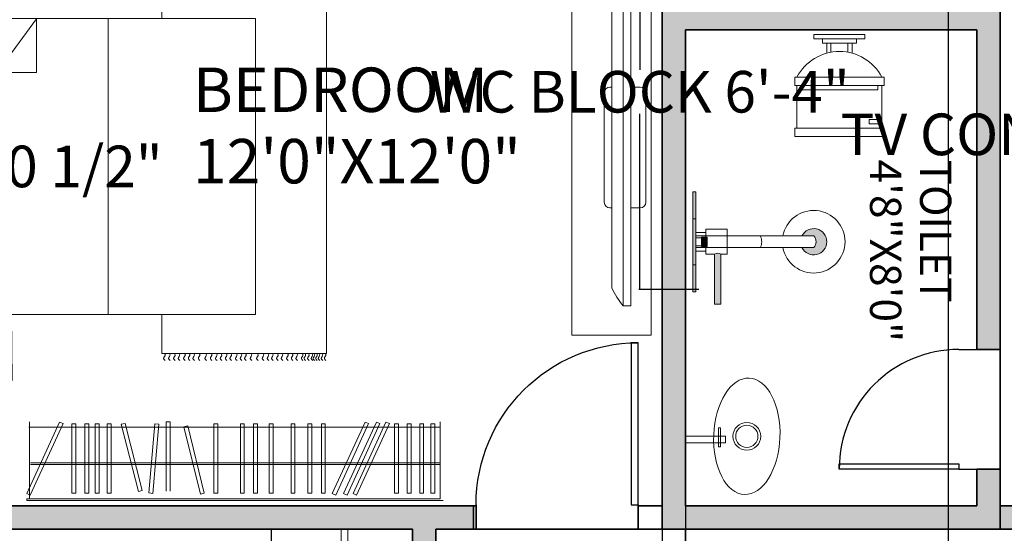
# Model space of a CAD drawing. Units: inches. Extents: x -4737294 to -4736756, y 1716389 to 1717040.
# Tile 20 of 25: x -4737186 to -4736996, y 1716844 to 1716943. Entities that reach past the tile are written whole.
import ezdxf

# ---------------------------------------------------------------- set-up
doc = ezdxf.new("R2010")
doc.units = ezdxf.units.IN
doc.header["$MEASUREMENT"] = 0
for name, color, linetype, lineweight in [('A-ANNO-DIMS', 2, 'Continuous', 18), ('A-AREA-IDEN', 250, 'Continuous', 18), ('A-WALL-PATT', 244, 'Continuous', 13), ('closet', 252, 'Continuous', 18), ('doors', 252, 'Continuous', 25), ('furniture', 250, 'Continuous', 18), ('PLUMBING FIXTURES', 252, 'Continuous', 18), ('walls', 252, 'Continuous', 35)]:
    doc.layers.add(name, color=color, linetype=linetype, lineweight=lineweight)
doc.styles.get("Standard").update_dxf_attribs({"font": 'arial.ttf'})
doc.dimstyles.get("Standard").update_dxf_attribs({"dimtxt": 8, "dimasz": 0.18, "dimexe": 0.18, "dimexo": 0.0625, "dimgap": 0.09, "dimtad": 0, "dimtih": 1, "dimtoh": 1, "dimzin": 0, "dimdsep": 46, "dimlunit": 3, "dimtxsty": 'Standard', "dimcen": 0.09, "dimadec": 0, "dimazin": 0, "dimtfac": 1, "dimtofl": 0, "dimtmove": 0, "dimatfit": 3, "dimfxl": 1, "dimtolj": 1, "dimtzin": 0, "dimarcsym": 0})

# ---------------------------------------------------------------- blocks, each defined once
blk = doc.blocks.new('CARPET')
at = {"layer": 'furniture'}
for p, q in [((-51.53, -98.11), (-51.53, -55.12)), ((-51.53, -55.12), (-41.27, -55.12)), ((36, -55.12), (51.55, -55.12)), ((51.55, -55.12), (51.55, -98.11)), ((51.55, -98.11), (-51.53, -98.11))]:
    blk.add_line(p, q, dxfattribs=at)
for points, knots in [([(-53.37, -55.99), (-53.22, -55.8), (-52.9, -55.41), (-52.34, -55.8), (-51.89, -56.08), (-51.65, -55.91), (-51.53, -55.83)], [0, 0, 0, 0, 0.653278, 1.290138, 1.740457, 2.114451, 2.114451, 2.114451, 2.114451]), ([(53.37, -55.99), (53.22, -55.8), (52.9, -55.41), (52.34, -55.8), (51.89, -56.08), (51.65, -55.91), (51.53, -55.83)], [0, 0, 0, 0, 0.653278, 1.290138, 1.740457, 2.114451, 2.114451, 2.114451, 2.114451]), ([(-53.37, -57.26), (-53.22, -57.07), (-52.9, -56.67), (-52.34, -57.07), (-51.89, -57.35), (-51.65, -57.17), (-51.53, -57.1)], [0, 0, 0, 0, 0.653278, 1.290138, 1.740457, 2.114451, 2.114451, 2.114451, 2.114451]), ([(-53.37, -58.59), (-53.22, -58.4), (-52.9, -58.01), (-52.34, -58.4), (-51.89, -58.68), (-51.65, -58.5), (-51.53, -58.43)], [0, 0, 0, 0, 0.653278, 1.290138, 1.740457, 2.114451, 2.114451, 2.114451, 2.114451]), ([(53.37, -57.26), (53.22, -57.07), (52.9, -56.67), (52.34, -57.07), (51.89, -57.35), (51.65, -57.17), (51.53, -57.1)], [0, 0, 0, 0, 0.653278, 1.290138, 1.740457, 2.114451, 2.114451, 2.114451, 2.114451]), ([(53.37, -58.59), (53.22, -58.4), (52.9, -58.01), (52.34, -58.4), (51.89, -58.68), (51.65, -58.5), (51.53, -58.43)], [0, 0, 0, 0, 0.653278, 1.290138, 1.740457, 2.114451, 2.114451, 2.114451, 2.114451]), ([(-53.37, -59.78), (-53.22, -59.58), (-52.9, -59.19), (-52.34, -59.58), (-51.89, -59.86), (-51.65, -59.69), (-51.53, -59.61)], [0, 0, 0, 0, 0.653278, 1.290138, 1.740457, 2.114451, 2.114451, 2.114451, 2.114451]), ([(-53.37, -61.22), (-53.22, -61.02), (-52.9, -60.63), (-52.34, -61.02), (-51.89, -61.3), (-51.65, -61.13), (-51.53, -61.05)], [0, 0, 0, 0, 0.653278, 1.290138, 1.740457, 2.114451, 2.114451, 2.114451, 2.114451]), ([(53.37, -59.78), (53.22, -59.58), (52.9, -59.19), (52.34, -59.58), (51.89, -59.86), (51.65, -59.69), (51.53, -59.61)], [0, 0, 0, 0, 0.653278, 1.290138, 1.740457, 2.114451, 2.114451, 2.114451, 2.114451]), ([(53.37, -61.22), (53.22, -61.02), (52.9, -60.63), (52.34, -61.02), (51.89, -61.3), (51.65, -61.13), (51.53, -61.05)], [0, 0, 0, 0, 0.653278, 1.290138, 1.740457, 2.114451, 2.114451, 2.114451, 2.114451]), ([(-53.37, -62.44), (-53.22, -62.25), (-52.9, -61.86), (-52.34, -62.25), (-51.89, -62.53), (-51.65, -62.36), (-51.53, -62.28)], [0, 0, 0, 0, 0.653278, 1.290138, 1.740457, 2.114451, 2.114451, 2.114451, 2.114451]), ([(-53.37, -63.63), (-53.22, -63.43), (-52.9, -63.04), (-52.34, -63.43), (-51.89, -63.72), (-51.65, -63.54), (-51.53, -63.46)], [0, 0, 0, 0, 0.653278, 1.290138, 1.740457, 2.114451, 2.114451, 2.114451, 2.114451]), ([(53.37, -62.44), (53.22, -62.25), (52.9, -61.86), (52.34, -62.25), (51.89, -62.53), (51.65, -62.36), (51.53, -62.28)], [0, 0, 0, 0, 0.653278, 1.290138, 1.740457, 2.114451, 2.114451, 2.114451, 2.114451]), ([(53.37, -63.63), (53.22, -63.43), (52.9, -63.04), (52.34, -63.43), (51.89, -63.72), (51.65, -63.54), (51.53, -63.46)], [0, 0, 0, 0, 0.653278, 1.290138, 1.740457, 2.114451, 2.114451, 2.114451, 2.114451]), ([(-53.37, -65.07), (-53.22, -64.87), (-52.9, -64.48), (-52.34, -64.87), (-51.89, -65.15), (-51.65, -64.98), (-51.53, -64.9)], [0, 0, 0, 0, 0.653278, 1.290138, 1.740457, 2.114451, 2.114451, 2.114451, 2.114451]), ([(-53.37, -66.76), (-53.22, -66.56), (-52.9, -66.17), (-52.34, -66.56), (-51.89, -66.84), (-51.65, -66.67), (-51.53, -66.59)], [0, 0, 0, 0, 0.653278, 1.290138, 1.740457, 2.114451, 2.114451, 2.114451, 2.114451]), ([(53.37, -65.07), (53.22, -64.87), (52.9, -64.48), (52.34, -64.87), (51.89, -65.15), (51.65, -64.98), (51.53, -64.9)], [0, 0, 0, 0, 0.653278, 1.290138, 1.740457, 2.114451, 2.114451, 2.114451, 2.114451]), ([(53.37, -66.76), (53.22, -66.56), (52.9, -66.17), (52.34, -66.56), (51.89, -66.84), (51.65, -66.67), (51.53, -66.59)], [0, 0, 0, 0, 0.653278, 1.290138, 1.740457, 2.114451, 2.114451, 2.114451, 2.114451]), ([(-53.37, -68.2), (-53.22, -68), (-52.9, -67.61), (-52.34, -68), (-51.89, -68.28), (-51.65, -68.11), (-51.53, -68.03)], [0, 0, 0, 0, 0.653278, 1.290138, 1.740457, 2.114451, 2.114451, 2.114451, 2.114451]), ([(-53.37, -69.53), (-53.22, -69.33), (-52.9, -68.94), (-52.34, -69.33), (-51.89, -69.61), (-51.65, -69.44), (-51.53, -69.36)], [0, 0, 0, 0, 0.653278, 1.290138, 1.740457, 2.114451, 2.114451, 2.114451, 2.114451]), ([(53.37, -68.2), (53.22, -68), (52.9, -67.61), (52.34, -68), (51.89, -68.28), (51.65, -68.11), (51.53, -68.03)], [0, 0, 0, 0, 0.653278, 1.290138, 1.740457, 2.114451, 2.114451, 2.114451, 2.114451]), ([(53.37, -69.53), (53.22, -69.33), (52.9, -68.94), (52.34, -69.33), (51.89, -69.61), (51.65, -69.44), (51.53, -69.36)], [0, 0, 0, 0, 0.653278, 1.290138, 1.740457, 2.114451, 2.114451, 2.114451, 2.114451]), ([(-53.37, -70.79), (-53.22, -70.6), (-52.9, -70.21), (-52.34, -70.6), (-51.89, -70.88), (-51.65, -70.7), (-51.53, -70.63)], [0, 0, 0, 0, 0.653278, 1.290138, 1.740457, 2.114451, 2.114451, 2.114451, 2.114451]), ([(-53.37, -72.12), (-53.22, -71.93), (-52.9, -71.54), (-52.34, -71.93), (-51.89, -72.21), (-51.65, -72.04), (-51.53, -71.96)], [0, 0, 0, 0, 0.653278, 1.290138, 1.740457, 2.114451, 2.114451, 2.114451, 2.114451]), ([(53.37, -70.79), (53.22, -70.6), (52.9, -70.21), (52.34, -70.6), (51.89, -70.88), (51.65, -70.7), (51.53, -70.63)], [0, 0, 0, 0, 0.653278, 1.290138, 1.740457, 2.114451, 2.114451, 2.114451, 2.114451]), ([(53.37, -72.12), (53.22, -71.93), (52.9, -71.54), (52.34, -71.93), (51.89, -72.21), (51.65, -72.04), (51.53, -71.96)], [0, 0, 0, 0, 0.653278, 1.290138, 1.740457, 2.114451, 2.114451, 2.114451, 2.114451]), ([(-53.37, -73.31), (-53.22, -73.11), (-52.9, -72.72), (-52.34, -73.11), (-51.89, -73.4), (-51.65, -73.22), (-51.53, -73.14)], [0, 0, 0, 0, 0.653278, 1.290138, 1.740457, 2.114451, 2.114451, 2.114451, 2.114451]), ([(-53.37, -74.75), (-53.22, -74.55), (-52.9, -74.16), (-52.34, -74.55), (-51.89, -74.83), (-51.65, -74.66), (-51.53, -74.58)], [0, 0, 0, 0, 0.653278, 1.290138, 1.740457, 2.114451, 2.114451, 2.114451, 2.114451]), ([(53.37, -73.31), (53.22, -73.11), (52.9, -72.72), (52.34, -73.11), (51.89, -73.4), (51.65, -73.22), (51.53, -73.14)], [0, 0, 0, 0, 0.653278, 1.290138, 1.740457, 2.114451, 2.114451, 2.114451, 2.114451]), ([(53.37, -74.75), (53.22, -74.55), (52.9, -74.16), (52.34, -74.55), (51.89, -74.83), (51.65, -74.66), (51.53, -74.58)], [0, 0, 0, 0, 0.653278, 1.290138, 1.740457, 2.114451, 2.114451, 2.114451, 2.114451]), ([(-53.37, -75.98), (-53.22, -75.78), (-52.9, -75.39), (-52.34, -75.78), (-51.89, -76.06), (-51.65, -75.89), (-51.53, -75.81)], [0, 0, 0, 0, 0.653278, 1.290138, 1.740457, 2.114451, 2.114451, 2.114451, 2.114451]), ([(-53.37, -77.16), (-53.22, -76.96), (-52.9, -76.57), (-52.34, -76.96), (-51.89, -77.25), (-51.65, -77.07), (-51.53, -76.99)], [0, 0, 0, 0, 0.653278, 1.290138, 1.740457, 2.114451, 2.114451, 2.114451, 2.114451]), ([(53.37, -75.98), (53.22, -75.78), (52.9, -75.39), (52.34, -75.78), (51.89, -76.06), (51.65, -75.89), (51.53, -75.81)], [0, 0, 0, 0, 0.653278, 1.290138, 1.740457, 2.114451, 2.114451, 2.114451, 2.114451]), ([(53.37, -77.16), (53.22, -76.96), (52.9, -76.57), (52.34, -76.96), (51.89, -77.25), (51.65, -77.07), (51.53, -76.99)], [0, 0, 0, 0, 0.653278, 1.290138, 1.740457, 2.114451, 2.114451, 2.114451, 2.114451]), ([(-53.37, -78.6), (-53.22, -78.4), (-52.9, -78.01), (-52.34, -78.4), (-51.89, -78.68), (-51.65, -78.51), (-51.53, -78.43)], [0, 0, 0, 0, 0.653278, 1.290138, 1.740457, 2.114451, 2.114451, 2.114451, 2.114451]), ([(53.37, -78.6), (53.22, -78.4), (52.9, -78.01), (52.34, -78.4), (51.89, -78.68), (51.65, -78.51), (51.53, -78.43)], [0, 0, 0, 0, 0.653278, 1.290138, 1.740457, 2.114451, 2.114451, 2.114451, 2.114451]), ([(-53.37, -80.29), (-53.22, -80.09), (-52.9, -79.7), (-52.34, -80.09), (-51.89, -80.37), (-51.65, -80.2), (-51.53, -80.12)], [0, 0, 0, 0, 0.653278, 1.290138, 1.740457, 2.114451, 2.114451, 2.114451, 2.114451]), ([(-53.37, -81.73), (-53.22, -81.53), (-52.9, -81.14), (-52.34, -81.53), (-51.89, -81.81), (-51.65, -81.64), (-51.53, -81.56)], [0, 0, 0, 0, 0.653278, 1.290138, 1.740457, 2.114451, 2.114451, 2.114451, 2.114451]), ([(53.37, -80.29), (53.22, -80.09), (52.9, -79.7), (52.34, -80.09), (51.89, -80.37), (51.65, -80.2), (51.53, -80.12)], [0, 0, 0, 0, 0.653278, 1.290138, 1.740457, 2.114451, 2.114451, 2.114451, 2.114451]), ([(53.37, -81.73), (53.22, -81.53), (52.9, -81.14), (52.34, -81.53), (51.89, -81.81), (51.65, -81.64), (51.53, -81.56)], [0, 0, 0, 0, 0.653278, 1.290138, 1.740457, 2.114451, 2.114451, 2.114451, 2.114451]), ([(-53.37, -83.06), (-53.22, -82.86), (-52.9, -82.47), (-52.34, -82.86), (-51.89, -83.14), (-51.65, -82.97), (-51.53, -82.89)], [0, 0, 0, 0, 0.653278, 1.290138, 1.740457, 2.114451, 2.114451, 2.114451, 2.114451]), ([(-53.37, -84.18), (-53.22, -83.99), (-52.9, -83.6), (-52.34, -83.99), (-51.89, -84.27), (-51.65, -84.09), (-51.53, -84.02)], [0, 0, 0, 0, 0.653278, 1.290138, 1.740457, 2.114451, 2.114451, 2.114451, 2.114451]), ([(53.37, -83.06), (53.22, -82.86), (52.9, -82.47), (52.34, -82.86), (51.89, -83.14), (51.65, -82.97), (51.53, -82.89)], [0, 0, 0, 0, 0.653278, 1.290138, 1.740457, 2.114451, 2.114451, 2.114451, 2.114451]), ([(53.37, -84.18), (53.22, -83.99), (52.9, -83.6), (52.34, -83.99), (51.89, -84.27), (51.65, -84.09), (51.53, -84.02)], [0, 0, 0, 0, 0.653278, 1.290138, 1.740457, 2.114451, 2.114451, 2.114451, 2.114451]), ([(-53.37, -85.51), (-53.22, -85.32), (-52.9, -84.93), (-52.34, -85.32), (-51.89, -85.6), (-51.65, -85.42), (-51.53, -85.35)], [0, 0, 0, 0, 0.653278, 1.290138, 1.740457, 2.114451, 2.114451, 2.114451, 2.114451]), ([(-53.37, -86.7), (-53.22, -86.5), (-52.9, -86.11), (-52.34, -86.5), (-51.89, -86.78), (-51.65, -86.61), (-51.53, -86.53)], [0, 0, 0, 0, 0.653278, 1.290138, 1.740457, 2.114451, 2.114451, 2.114451, 2.114451]), ([(53.37, -85.51), (53.22, -85.32), (52.9, -84.93), (52.34, -85.32), (51.89, -85.6), (51.65, -85.42), (51.53, -85.35)], [0, 0, 0, 0, 0.653278, 1.290138, 1.740457, 2.114451, 2.114451, 2.114451, 2.114451]), ([(53.37, -86.7), (53.22, -86.5), (52.9, -86.11), (52.34, -86.5), (51.89, -86.78), (51.65, -86.61), (51.53, -86.53)], [0, 0, 0, 0, 0.653278, 1.290138, 1.740457, 2.114451, 2.114451, 2.114451, 2.114451]), ([(-53.37, -88.14), (-53.22, -87.94), (-52.9, -87.55), (-52.34, -87.94), (-51.89, -88.22), (-51.65, -88.05), (-51.53, -87.97)], [0, 0, 0, 0, 0.653278, 1.290138, 1.740457, 2.114451, 2.114451, 2.114451, 2.114451]), ([(-53.37, -89.36), (-53.22, -89.17), (-52.9, -88.78), (-52.34, -89.17), (-51.89, -89.45), (-51.65, -89.28), (-51.53, -89.2)], [0, 0, 0, 0, 0.653278, 1.290138, 1.740457, 2.114451, 2.114451, 2.114451, 2.114451]), ([(53.37, -88.14), (53.22, -87.94), (52.9, -87.55), (52.34, -87.94), (51.89, -88.22), (51.65, -88.05), (51.53, -87.97)], [0, 0, 0, 0, 0.653278, 1.290138, 1.740457, 2.114451, 2.114451, 2.114451, 2.114451]), ([(53.37, -89.36), (53.22, -89.17), (52.9, -88.78), (52.34, -89.17), (51.89, -89.45), (51.65, -89.28), (51.53, -89.2)], [0, 0, 0, 0, 0.653278, 1.290138, 1.740457, 2.114451, 2.114451, 2.114451, 2.114451]), ([(-53.37, -90.55), (-53.22, -90.35), (-52.9, -89.96), (-52.34, -90.35), (-51.89, -90.64), (-51.65, -90.46), (-51.53, -90.38)], [0, 0, 0, 0, 0.653278, 1.290138, 1.740457, 2.114451, 2.114451, 2.114451, 2.114451]), ([(-53.37, -91.99), (-53.22, -91.79), (-52.9, -91.4), (-52.34, -91.79), (-51.89, -92.07), (-51.65, -91.9), (-51.53, -91.82)], [0, 0, 0, 0, 0.653278, 1.290138, 1.740457, 2.114451, 2.114451, 2.114451, 2.114451]), ([(-53.37, -92.69), (-53.22, -92.48), (-52.9, -92.08), (-52.35, -92.49), (-51.89, -92.77), (-51.65, -92.6), (-51.53, -92.52)], [0, 0, 0, 0, 0.663904, 1.307406, 1.757725, 2.131719, 2.131719, 2.131719, 2.131719]), ([(53.37, -90.55), (53.22, -90.35), (52.9, -89.96), (52.34, -90.35), (51.9, -90.63), (51.66, -90.47), (51.55, -90.4)], [0, 0, 0, 0, 0.653278, 1.290138, 1.740457, 2.0926, 2.0926, 2.0926, 2.0926]), ([(53.37, -91.99), (53.22, -91.79), (52.9, -91.4), (52.34, -91.79), (51.9, -92.07), (51.66, -91.91), (51.55, -91.83)], [0, 0, 0, 0, 0.653278, 1.290138, 1.740457, 2.0926, 2.0926, 2.0926, 2.0926]), ([(53.37, -92.69), (53.22, -92.49), (52.9, -92.09), (52.34, -92.49), (51.9, -92.77), (51.66, -92.61), (51.55, -92.53)], [0, 0, 0, 0, 0.656792, 1.295826, 1.746145, 2.098292, 2.098292, 2.098292, 2.098292]), ([(-53.37, -93.61), (-53.22, -93.42), (-52.9, -93.03), (-52.34, -93.42), (-51.89, -93.7), (-51.65, -93.52), (-51.53, -93.45)], [0, 0, 0, 0, 0.653278, 1.290138, 1.740457, 2.114451, 2.114451, 2.114451, 2.114451]), ([(-53.37, -94.55), (-53.22, -94.35), (-52.9, -93.96), (-52.34, -94.35), (-51.89, -94.63), (-51.65, -94.46), (-51.53, -94.38)], [0, 0, 0, 0, 0.653278, 1.290138, 1.740457, 2.114451, 2.114451, 2.114451, 2.114451]), ([(-53.37, -95.05), (-53.22, -94.85), (-52.9, -94.46), (-52.34, -94.85), (-51.89, -95.14), (-51.65, -94.96), (-51.53, -94.88)], [0, 0, 0, 0, 0.653278, 1.290138, 1.740457, 2.114451, 2.114451, 2.114451, 2.114451]), ([(53.37, -93.66), (53.22, -93.46), (52.9, -93.07), (52.34, -93.46), (51.9, -93.74), (51.66, -93.58), (51.55, -93.5)], [0, 0, 0, 0, 0.653278, 1.290138, 1.740457, 2.0926, 2.0926, 2.0926, 2.0926]), ([(53.37, -94.59), (53.22, -94.4), (52.9, -94.01), (52.34, -94.4), (51.9, -94.68), (51.66, -94.51), (51.55, -94.44)], [0, 0, 0, 0, 0.653278, 1.290138, 1.740457, 2.0926, 2.0926, 2.0926, 2.0926]), ([(53.37, -95.1), (53.22, -94.9), (52.9, -94.51), (52.34, -94.9), (51.9, -95.18), (51.66, -95.02), (51.55, -94.94)], [0, 0, 0, 0, 0.653278, 1.290138, 1.740457, 2.0926, 2.0926, 2.0926, 2.0926]), ([(-53.37, -95.73), (-53.22, -95.54), (-52.9, -95.15), (-52.34, -95.54), (-51.89, -95.82), (-51.65, -95.65), (-51.53, -95.57)], [0, 0, 0, 0, 0.653278, 1.290138, 1.740457, 2.114451, 2.114451, 2.114451, 2.114451]), ([(-53.37, -96.38), (-53.22, -96.18), (-52.9, -95.79), (-52.34, -96.18), (-51.89, -96.47), (-51.65, -96.29), (-51.53, -96.21)], [0, 0, 0, 0, 0.653278, 1.290138, 1.740457, 2.114451, 2.114451, 2.114451, 2.114451]), ([(-53.37, -97.17), (-53.22, -96.98), (-52.9, -96.59), (-52.34, -96.98), (-51.89, -97.26), (-51.65, -97.08), (-51.53, -97.01)], [0, 0, 0, 0, 0.653278, 1.290138, 1.740457, 2.114451, 2.114451, 2.114451, 2.114451]), ([(-53.37, -97.99), (-53.22, -97.79), (-52.9, -97.4), (-52.34, -97.79), (-51.89, -98.08), (-51.65, -97.9), (-51.53, -97.82)], [0, 0, 0, 0, 0.653278, 1.290138, 1.740457, 2.114451, 2.114451, 2.114451, 2.114451]), ([(53.37, -95.78), (53.22, -95.58), (52.9, -95.19), (52.34, -95.58), (51.89, -95.86), (51.65, -95.69), (51.53, -95.61)], [0, 0, 0, 0, 0.653278, 1.290138, 1.740457, 2.114451, 2.114451, 2.114451, 2.114451]), ([(53.37, -96.43), (53.22, -96.23), (52.9, -95.84), (52.34, -96.23), (51.89, -96.51), (51.65, -96.34), (51.53, -96.26)], [0, 0, 0, 0, 0.653278, 1.290138, 1.740457, 2.114451, 2.114451, 2.114451, 2.114451]), ([(53.37, -97.22), (53.22, -97.02), (52.9, -96.63), (52.34, -97.02), (51.89, -97.3), (51.65, -97.13), (51.53, -97.05)], [0, 0, 0, 0, 0.653278, 1.290138, 1.740457, 2.114451, 2.114451, 2.114451, 2.114451]), ([(53.37, -97.99), (53.22, -97.79), (52.9, -97.4), (52.34, -97.79), (51.89, -98.08), (51.65, -97.9), (51.53, -97.82)], [0, 0, 0, 0, 0.653278, 1.290138, 1.740457, 2.114451, 2.114451, 2.114451, 2.114451])]:
    blk.add_open_spline(points, degree=3, knots=knots, dxfattribs=at)
blk = doc.blocks.new('A$C58D270C6')
at = {"layer": 'furniture'}
for p, q in [((9.09, 124.13), (9.09, 108.87)), ((1.46, 116.5), (16.73, 116.5)), ((14.97, 94.84), (24.62, 107.92)), ((24.62, 94.93), (24.62, 107.92)), ((42.08, 108), (42.08, 36)), ((14.97, 94.93), (24.62, 94.93)), ((14.97, 94.84), (14.97, 36)), ((16.22, 94.93), (16.22, 36)), ((9.25, 36), (9.25, 20.74)), ((1.62, 28.37), (16.88, 28.37))]:
    blk.add_line(p, q, dxfattribs=at)
for points in [[(18.5, 108), (18.34, 124.13), (-0.16, 124.13), (0, 108)], [(0, 108), (77.91, 108), (77.91, 36), (0, 36)], [(4.09, 94.93), (14.97, 94.93), (14.97, 73.83), (4.09, 73.83)], [(4.09, 65.23), (14.97, 65.23), (14.97, 44.13), (4.09, 44.13)], [(18.65, 19.87), (18.5, 36), (0, 36), (0.16, 19.87)]]:
    blk.add_lwpolyline(points, close=True, dxfattribs=at)
for centre in [(9.09, 116.5), (9.25, 28.37)]:
    blk.add_circle(centre, 5.95, dxfattribs=at)
at = {"layer": 'furniture', "xscale": 0.9312884925094044, "yscale": 0.9312884925094044, "zscale": 0.9312884925094044, "rotation": 90}
blk.add_blockref('CARPET', (3.79, 74.47), dxfattribs=at)
blk = doc.blocks.new('closet')
at = {"layer": 'closet'}
for p, q in [((-0.71, -5.58), (5.59, 8.19)), ((6.27, 7.88), (-0.04, -5.89)), ((5.59, 8.19), (6.27, 7.88)), ((7.92, 7.84), (8.68, 7.84)), ((7.92, 7.84), (7.92, -5.51)), ((8.68, 7.84), (8.68, -5.51)), ((10.44, 7.84), (11.2, 7.84)), ((10.44, 7.84), (10.44, -5.51)), ((11.2, 7.84), (11.2, -5.51)), ((12.45, 7.84), (13.21, 7.84)), ((12.45, 7.84), (12.45, -5.51)), ((13.21, 7.84), (13.21, -5.51)), ((14.71, 7.84), (15.47, 7.84)), ((14.71, 7.84), (14.71, -5.51)), ((15.47, 7.84), (15.47, -5.51)), ((17.44, 7.75), (18.17, 7.93)), ((17.44, 7.75), (20.73, -5.2)), ((18.17, 7.93), (21.46, -5.01)), ((23.92, 7.84), (22.75, -5.46)), ((24.67, 7.78), (23.51, -5.53)), ((23.92, 7.84), (24.67, 7.78)), ((26.09, 8.25), (26.09, -5.1)), ((26.84, 8.25), (26.84, -5.1)), ((35.23, 7.84), (35.23, -5.51)), ((35.99, 7.84), (35.99, -5.51)), ((40.33, 7.84), (40.33, -5.51)), ((41.08, 7.84), (41.08, -5.51)), ((42.85, 7.84), (42.85, -5.51)), ((43.61, 7.84), (43.61, -5.51)), ((45.9, 7.84), (45.9, -5.51)), ((46.65, 7.84), (46.65, -5.51)), ((50.07, 7.84), (50.07, -5.51)), ((50.82, 7.84), (50.82, -5.51)), ((53.32, 7.84), (53.32, -5.51)), ((54.08, 7.84), (54.08, -5.51)), ((55.9, 7.84), (55.9, -5.51)), ((56.65, 7.84), (56.65, -5.51)), ((57.99, -5.58), (64.3, 8.19)), ((64.97, 7.88), (58.67, -5.89)), ((60.19, -5.58), (66.49, 8.19)), ((67.17, 7.88), (60.87, -5.89)), ((62, -5.58), (68.3, 8.19)), ((68.98, 7.88), (62.67, -5.89)), ((69.96, 7.84), (69.96, -5.51)), ((70.72, 7.84), (70.72, -5.51)), ((72.43, 7.84), (72.43, -5.51)), ((73.19, 7.84), (73.19, -5.51)), ((74.82, 7.84), (74.82, -5.51)), ((75.57, 7.84), (75.57, -5.51)), ((76.94, 7.84), (76.94, -5.51)), ((77.69, 7.84), (77.69, -5.51)), ((-0.23, 7.39), (-0.23, -6.57)), ((29.49, 7.29), (32.64, -5.69)), ((30.22, 7.46), (33.37, -5.51)), ((56.23, 0.33), (0, 0.33)), ((56.2, 0), (0, 0)), ((56.2, 0), (78.76, 0)), ((56.23, 0.33), (78.76, 0.33)), ((-0.04, -5.89), (-0.71, -5.58)), ((21.46, -5.01), (20.73, -5.2)), ((23.51, -5.53), (22.75, -5.46)), ((33.37, -5.51), (32.64, -5.69)), ((35.99, -5.51), (35.23, -5.51)), ((41.08, -5.51), (40.33, -5.51)), ((43.61, -5.51), (42.85, -5.51)), ((46.65, -5.51), (45.9, -5.51)), ((50.82, -5.51), (50.07, -5.51)), ((54.08, -5.51), (53.32, -5.51)), ((56.65, -5.51), (55.9, -5.51)), ((58.67, -5.89), (57.99, -5.58)), ((60.87, -5.89), (60.19, -5.58)), ((62.67, -5.89), (62, -5.58)), ((70.72, -5.51), (69.96, -5.51)), ((73.19, -5.51), (72.43, -5.51)), ((75.57, -5.51), (74.82, -5.51)), ((77.69, -5.51), (76.94, -5.51))]:
    blk.add_line(p, q, dxfattribs=at)
blk = doc.blocks.new('rotated closet')
at = {"layer": 'closet'}
for p, q in [((26.32, 0.86), (27.07, 0.86)), ((29.72, -0.11), (30.45, 0.07)), ((35.46, 0.45), (36.22, 0.45)), ((40.56, 0.45), (41.31, 0.45)), ((43.08, 0.45), (43.84, 0.45)), ((46.13, 0.45), (46.88, 0.45)), ((50.3, 0.45), (51.05, 0.45)), ((53.56, 0.45), (54.31, 0.45)), ((56.13, 0.45), (56.88, 0.45)), ((64.53, 0.8), (65.2, 0.49)), ((66.72, 0.8), (67.4, 0.49)), ((68.53, 0.8), (69.21, 0.49)), ((70.19, 0.45), (70.95, 0.45)), ((72.66, 0.45), (73.42, 0.45)), ((75.05, 0.45), (75.81, 0.45)), ((77.17, 0.45), (77.92, 0.45)), ((78.99, 0), (78.99, -13.96)), ((8.91, -12.91), (8.15, -12.91)), ((11.43, -12.91), (10.67, -12.91)), ((13.44, -12.91), (12.68, -12.91)), ((15.7, -12.91), (14.94, -12.91)), ((-0.46, -14.27), (79.54, -14.27)), ((0, -13.96), (78.99, -13.96))]:
    blk.add_line(p, q, dxfattribs=at)
blk.add_blockref('closet', (0.23, -7.39), dxfattribs=at)
blk = doc.blocks.new('O.H SHOWER-PL')
at = {"layer": 'PLUMBING FIXTURES'}
for points in [[(-1.838, 0), (-1.838, -0.25), (1.838, -0.25), (1.838, 0)], [(0.461, -8.724), (0.461, -9.667, -0.422337), (-0.461, -9.667), (-0.461, -8.724, 4.325472)]]:
    blk.add_hatch(color=256, dxfattribs=at).paths.add_polyline_path(points)
for p, q in [((-1.838, 0), (-1.838, -0.25)), ((1.838, 0), (-1.838, 0)), ((1.838, 0), (1.838, -0.25)), ((1.838, -0.25), (-1.838, -0.25)), ((-0.461, -0.25), (-0.461, -9.667)), ((0.461, -0.25), (0.461, -9.667))]:
    blk.add_line(p, q, dxfattribs=at)
for centre, radius, start, end in [((0, -4.479), 1.033, 243.52996, 296.47004), ((0, -9.667), 2.501, 100.61004, 79.38997), ((0, -9.667), 1.049, 116.03487, 63.96515), ((0, -9.219), 0.643, 224.20776, 315.79224)]:
    blk.add_arc(centre, radius, start, end, dxfattribs=at)
blk = doc.blocks.new('DIVERTER-PL')
at = {"layer": 'PLUMBING FIXTURES'}
for points in [[(4, 0), (-4, 0), (-4, -0.25), (4, -0.25)], [(0.375, -1.144), (0.375, -0.704), (-0.375, -0.704), (-0.375, -1.144)], [(1, -1.751, 0.30818), (1, -2.251), (5, -2.251), (5, -1.751)]]:
    blk.add_hatch(color=256, dxfattribs=at).paths.add_polyline_path(points)
for p, q in [((-4, 0), (-4, -0.25)), ((-4, 0), (4, 0)), ((4, 0), (4, -0.25)), ((-4, -0.25), (4, -0.25)), ((-4, -0.25), (4, -0.25)), ((-0.75, -0.25), (-0.75, -1.05)), ((-0.375, -0.704), (0.375, -0.704)), ((-0.375, -0.704), (-0.375, -1.144)), ((-0.318, -0.704), (-0.318, -0.25)), ((0.318, -0.704), (0.318, -0.25)), ((0.375, -0.704), (0.375, -1.144)), ((0.75, -0.25), (0.75, -1.05)), ((-1, -1.05), (-0.375, -1.05)), ((-1, -1.05), (-1, -2.75)), ((-0.375, -1.144), (0.375, -1.144)), ((0.375, -1.05), (1, -1.05)), ((1, -1.05), (1, -1.751)), ((1, -2.251), (1, -2.75)), ((-1, -2.75), (1, -2.75))]:
    blk.add_line(p, q, dxfattribs=at)
at = {"layer": 'PLUMBING FIXTURES', "ltscale": 12}
for p, q in [((1, -1.751), (5, -1.751)), ((1, -2.251), (5, -2.251)), ((5, -2.251), (5, -1.751))]:
    blk.add_line(p, q, dxfattribs=at)
at = {"layer": 'PLUMBING FIXTURES'}
blk.add_arc((1.367, -2.001), 0.444, 145.74346, 214.25654, dxfattribs=at)
blk = doc.blocks.new('A$C7F153053')
at = {"layer": 'PLUMBING FIXTURES', "xscale": -1, "rotation": 270}
for name in ['DIVERTER-PL', 'O.H SHOWER-PL']:
    blk.add_blockref(name, (12.166, 4), dxfattribs=at)
blk = doc.blocks.new('Toilet - Imperial')
for p, q in [((-10, 22), (-10, 12)), ((-10, 21), (-7, 21)), ((-7, 21), (-7, 20)), ((10, 12), (10, 22)), ((-7, 20), (-10, 20)), ((10.5, 12), (-10.5, 12)), ((-10.5, 10), (-10.5, 12)), ((9, 13), (-9, 13)), ((-9, 13), (-9, 12)), ((9, 12), (9, 13)), ((10.5, 12), (10.5, 10)), ((10.5, 10), (-10.5, 10)), ((-3, 4.4065), (-3, 2)), ((-2, 2), (-2, 4.1658)), ((2, 4.1658), (2, 2)), ((3, 2), (3, 4.4065)), ((4, 2), (-4, 2)), ((-4, 2), (-4, 1)), ((4, 1), (4, 2))]:
    blk.add_line(p, q)
for points in [[(10.5, 22), (10.5, 24), (-10.5, 24), (-10.5, 22)], [(6, 0), (6, 1), (-6, 1), (-6, 0)]]:
    blk.add_lwpolyline(points, close=True)
blk.add_arc((0, 15.3333), 11.3333, 208.0725, 331.9275)
blk = doc.blocks.new('*U20')
for p, q in [((0, 0), (0, -6)), ((40, 0), (40, -6))]:
    blk.add_line(p, q)
blk.add_lwpolyline([(0, 0), (0, 40), (1.75, 40), (1.75, 0)], close=True)
blk.add_arc((0, 0), 40, 0, 90)
blk = doc.blocks.new('LAVATORY-OVAL-WITH-TAP')
for p, q in [((6.3, 12.81), (6.3, 9.15)), ((6.71, 12.81), (6.3, 12.81)), ((6.71, 9.15), (6.71, 12.81)), ((0, 11.19), (7.64, 11.19)), ((7.64, 9.95), (0, 9.95)), ((7.64, 11.19), (7.64, 9.95)), ((6.3, 9.15), (6.71, 9.15))]:
    blk.add_line(p, q)
for radius in [2.67, 2.13, 2.13, 2.13]:
    blk.add_circle((11.77, 11.19), radius)
blk.add_ellipse((11.77, 11.19), major_axis=(-0.46, -11.19), ratio=0.56899)
blk = doc.blocks.new('PLASMA-LARGE')
at = {"layer": 'furniture'}
for p, q in [((-7.26, 0), (7.26, 0)), ((-18.61, -1), (18.61, -1)), ((-8, -1), (-8, -0.74)), ((8, -1), (8, -0.74)), ((-21, -2.5), (21, -2.5)), ((-21, -2.5), (-21, -3.5)), ((21, -2.5), (21, -3.5)), ((-21, -3.5), (21, -3.5)), ((-8, -3.5), (-8, -4.76)), ((8, -3.5), (8, -4.76)), ((-7.26, -5.5), (7.26, -5.5))]:
    blk.add_line(p, q, dxfattribs=at)
for centre, radius, start, end in [((-7.26, -0.74), 0.744, 90, 180), ((7.26, -0.74), 0.744, 0, 90), ((-13.97, -11.05), 11.07, 114.7602, 129.4175), ((13.97, -11.05), 11.07, 50.5825, 65.2398), ((-7.26, -4.76), 0.744, 180, 270), ((7.26, -4.76), 0.744, 270, 0)]:
    blk.add_arc(centre, radius, start, end, dxfattribs=at)
blk = doc.blocks.new('TV-CONSOLE-BEDROOM')
for p, q in [((15.21, 71.77), (0, 71.77)), ((0, 71.77), (0, 0)), ((15.21, 0), (15.21, 71.77)), ((0, 0), (15.21, 0))]:
    blk.add_line(p, q)
at = {"xscale": 1.450199298177205, "yscale": 1.450199298177205, "zscale": 1.450199298177205, "rotation": 90}
blk.add_blockref('PLASMA-LARGE', (6.22, 36.13), dxfattribs=at)
blk = doc.blocks.new('*D31')
at = {"layer": 'A-ANNO-DIMS', "color": 0, "lineweight": -2, "transparency": 16777216}
for p, q in [((-4737202.03, 1716955.51), (-4737214.51, 1716955.51)), ((-4737214.33, 1716955.33), (-4737214.33, 1716918.54)), ((-4737214.33, 1716873.3), (-4737214.33, 1716910.08)), ((-4737202.03, 1716873.12), (-4737214.51, 1716873.12))]:
    blk.add_line(p, q, dxfattribs=at)
at = {"layer": 'A-ANNO-DIMS', "color": 0, "transparency": 16777216}
for points in [[(-4737214.36, 1716955.33), (-4737214.3, 1716955.33), (-4737214.33, 1716955.51)], [(-4737214.36, 1716873.3), (-4737214.3, 1716873.3), (-4737214.33, 1716873.12)]]:
    blk.add_solid(points, dxfattribs=at)
at = {"layer": 'Defpoints', "color": 0, "transparency": 16777216}
for p in [(-4737214.33, 1716955.51), (-4737201.97, 1716955.51), (-4737201.97, 1716873.12)]:
    blk.add_point(p, dxfattribs=at)
at = {"layer": 'A-ANNO-DIMS', "color": 0, "transparency": 16777216, "insert": (-4737214.33, 1716914.31), "char_height": 8, "attachment_point": 5}
blk.add_mtext('\\A1;BED GROUP 6\'-10 1/2"', dxfattribs=at)
blk = doc.blocks.new('*D39')
at = {"layer": 'A-ANNO-DIMS', "color": 0, "lineweight": -2, "transparency": 16777216}
for p, q in [((-4737055.1, 1716966.68), (-4737066.63, 1716966.68)), ((-4737066.45, 1716966.5), (-4737066.45, 1716932.89)), ((-4737066.45, 1716890.83), (-4737066.45, 1716924.44)), ((-4737055.1, 1716890.65), (-4737066.63, 1716890.65))]:
    blk.add_line(p, q, dxfattribs=at)
at = {"layer": 'A-ANNO-DIMS', "color": 0, "transparency": 16777216}
for points in [[(-4737066.48, 1716966.5), (-4737066.42, 1716966.5), (-4737066.45, 1716966.68)], [(-4737066.48, 1716890.83), (-4737066.42, 1716890.83), (-4737066.45, 1716890.65)]]:
    blk.add_solid(points, dxfattribs=at)
at = {"layer": 'Defpoints', "color": 0, "transparency": 16777216}
for p in [(-4737055.04, 1716966.68), (-4737066.45, 1716890.65), (-4737055.04, 1716890.65)]:
    blk.add_point(p, dxfattribs=at)
at = {"layer": 'A-ANNO-DIMS', "color": 0, "transparency": 16777216, "insert": (-4737066.45, 1716928.67), "char_height": 8, "attachment_point": 5}
blk.add_mtext('\\A1;WC BLOCK 6\'-4"', dxfattribs=at)
blk = doc.blocks.new('*D41')
at = {"layer": 'A-ANNO-DIMS', "color": 0, "lineweight": -2, "transparency": 16777216}
for p, q in [((-4737133.94, 1716826.11), (-4737133.94, 1716822.59)), ((-4737111.26, 1716826.11), (-4737111.26, 1716822.59)), ((-4737133.76, 1716822.77), (-4737111.44, 1716822.77)), ((-4737111.26, 1716822.77), (-4737111.08, 1716822.77))]:
    blk.add_line(p, q, dxfattribs=at)
at = {"layer": 'A-ANNO-DIMS', "color": 0, "transparency": 16777216}
for points in [[(-4737133.76, 1716822.8), (-4737133.76, 1716822.74), (-4737133.94, 1716822.77)], [(-4737111.44, 1716822.8), (-4737111.44, 1716822.74), (-4737111.26, 1716822.77)]]:
    blk.add_solid(points, dxfattribs=at)
at = {"layer": 'Defpoints', "color": 0, "transparency": 16777216}
for p in [(-4737133.94, 1716826.17), (-4737111.26, 1716826.17), (-4737111.26, 1716822.77)]:
    blk.add_point(p, dxfattribs=at)
at = {"layer": 'A-ANNO-DIMS', "color": 0, "transparency": 16777216, "insert": (-4737056.03, 1716822.77), "char_height": 8, "attachment_point": 5}
blk.add_mtext('\\A1;BASIN 1\'-10 1/2" TYP.', dxfattribs=at)
blk = doc.blocks.new('*D42')
at = {"layer": 'A-ANNO-DIMS', "color": 0, "lineweight": -2, "transparency": 16777216}
for p, q in [((-4737134, 1716844.56), (-4737137.52, 1716844.56)), ((-4737137.34, 1716844.38), (-4737137.34, 1716839.59)), ((-4737137.34, 1716826.35), (-4737137.34, 1716831.14)), ((-4737134, 1716826.17), (-4737137.52, 1716826.17))]:
    blk.add_line(p, q, dxfattribs=at)
at = {"layer": 'A-ANNO-DIMS', "color": 0, "transparency": 16777216}
for points in [[(-4737137.37, 1716844.38), (-4737137.31, 1716844.38), (-4737137.34, 1716844.56)], [(-4737137.37, 1716826.35), (-4737137.31, 1716826.35), (-4737137.34, 1716826.17)]]:
    blk.add_solid(points, dxfattribs=at)
at = {"layer": 'Defpoints', "color": 0, "transparency": 16777216}
for p in [(-4737133.94, 1716844.56), (-4737137.34, 1716826.17), (-4737133.94, 1716826.17)]:
    blk.add_point(p, dxfattribs=at)
at = {"layer": 'A-ANNO-DIMS', "color": 0, "transparency": 16777216, "insert": (-4737137.34, 1716835.37), "char_height": 8, "attachment_point": 5}
blk.add_mtext('\\A1;1\'-6 1/2" TYP.', dxfattribs=at)
blk = doc.blocks.new('*D43')
at = {"layer": 'A-ANNO-DIMS', "color": 0, "lineweight": -2, "transparency": 16777216}
for p, q in [((-4736980.34, 1716956.36), (-4736969.46, 1716956.36)), ((-4736969.64, 1716956.18), (-4736969.64, 1716924.7)), ((-4736969.64, 1716884.77), (-4736969.64, 1716916.25)), ((-4736980.34, 1716884.59), (-4736969.46, 1716884.59))]:
    blk.add_line(p, q, dxfattribs=at)
at = {"layer": 'A-ANNO-DIMS', "color": 0, "transparency": 16777216}
for points in [[(-4736969.67, 1716956.18), (-4736969.61, 1716956.18), (-4736969.64, 1716956.36)], [(-4736969.67, 1716884.77), (-4736969.61, 1716884.77), (-4736969.64, 1716884.59)]]:
    blk.add_solid(points, dxfattribs=at)
at = {"layer": 'Defpoints', "color": 0, "transparency": 16777216}
for p in [(-4736980.4, 1716956.36), (-4736969.64, 1716956.36), (-4736980.4, 1716884.59)]:
    blk.add_point(p, dxfattribs=at)
at = {"layer": 'A-ANNO-DIMS', "color": 0, "transparency": 16777216, "insert": (-4736969.64, 1716920.48), "char_height": 8, "attachment_point": 5}
blk.add_mtext('\\A1;TV CONSOLE 6\'-0" TYP.', dxfattribs=at)
blk = doc.blocks.new('*D62')
at = {"layer": 'A-ANNO-DIMS', "color": 0, "lineweight": -2, "transparency": 16777216}
for p, q in [((-4737062.14, 1716849), (-4737062.14, 1716423.69)), ((-4737057.64, 1716849), (-4737057.64, 1716423.69)), ((-4737061.96, 1716423.87), (-4737057.82, 1716423.87)), ((-4737057.64, 1716423.87), (-4737057.46, 1716423.87))]:
    blk.add_line(p, q, dxfattribs=at)
at = {"layer": 'A-ANNO-DIMS', "color": 0, "transparency": 16777216}
for points in [[(-4737061.96, 1716423.9), (-4737061.96, 1716423.84), (-4737062.14, 1716423.87)], [(-4737057.82, 1716423.9), (-4737057.82, 1716423.84), (-4737057.64, 1716423.87)]]:
    blk.add_solid(points, dxfattribs=at)
at = {"layer": 'Defpoints', "color": 0, "transparency": 16777216}
for p in [(-4737062.14, 1716849.06), (-4737057.64, 1716849.06), (-4737057.64, 1716423.87)]:
    blk.add_point(p, dxfattribs=at)
at = {"layer": 'A-ANNO-DIMS', "color": 0, "transparency": 16777216, "insert": (-4737037.42, 1716423.87), "char_height": 8, "attachment_point": 5}
blk.add_mtext('\\A1;0\'-4 1/2"', dxfattribs=at)
blk = doc.blocks.new('*D65')
at = {"layer": 'A-ANNO-DIMS', "color": 0, "lineweight": -2, "transparency": 16777216}
for p, q in [((-4737007.1, 1716596.13), (-4737007.1, 1717035.24)), ((-4737006.92, 1717035.06), (-4736984.27, 1717035.06)), ((-4736984.09, 1716596.13), (-4736984.09, 1717035.24)), ((-4736984.09, 1717035.06), (-4736983.91, 1717035.06))]:
    blk.add_line(p, q, dxfattribs=at)
at = {"layer": 'A-ANNO-DIMS', "color": 0, "transparency": 16777216}
for points in [[(-4737006.92, 1717035.09), (-4737006.92, 1717035.03), (-4737007.1, 1717035.06)], [(-4736984.27, 1717035.09), (-4736984.27, 1717035.03), (-4736984.09, 1717035.06)]]:
    blk.add_solid(points, dxfattribs=at)
at = {"layer": 'Defpoints', "color": 0, "transparency": 16777216}
for p in [(-4736984.09, 1717035.06), (-4737007.1, 1716596.06), (-4736984.09, 1716596.06)]:
    blk.add_point(p, dxfattribs=at)
at = {"layer": 'A-ANNO-DIMS', "color": 0, "transparency": 16777216, "insert": (-4736970.46, 1717035.06), "char_height": 8, "attachment_point": 5}
blk.add_mtext('\\A1;1\'-11"', dxfattribs=at)

msp = doc.modelspace()

# ---------------------------------------------------------------- hatches: boundary and pattern name
at = {"layer": 'A-WALL-PATT'}
h = msp.add_hatch(color=256, dxfattribs=at)
h.dxf.hatch_style = 1
h.paths.add_polyline_path([(-4737206.144, 1716844.565), (-4737110.144, 1716844.565), (-4737110.144, 1716823.907), (-4737105.644, 1716823.907), (-4737105.644, 1716844.565), (-4737098.44, 1716844.565), (-4737098.44, 1716849.065), (-4737206.144, 1716849.065), (-4737206.144, 1716993.065), (-4736864.144, 1716993.065), (-4736864.144, 1716849.065), (-4736963.275, 1716849.065), (-4736994.446, 1716849.065), (-4736997.144, 1716849.065), (-4736997.144, 1716844.565), (-4736864.144, 1716844.565), (-4736864.144, 1716668.565), (-4736934.391, 1716668.565), (-4736934.391, 1716664.065), (-4736864.144, 1716664.065), (-4736864.144, 1716462.065), (-4736855.144, 1716462.065), (-4736855.144, 1717002.065), (-4737215.144, 1717002.065), (-4737215.144, 1716462.065), (-4737206.144, 1716462.065), (-4737206.144, 1716659.065), (-4737062.144, 1716659.065), (-4737062.144, 1716647.493), (-4737057.644, 1716647.493), (-4737057.644, 1716796.565), (-4737071.812, 1716796.565), (-4737071.812, 1716792.065), (-4737070.805, 1716792.065), (-4737062.144, 1716792.065), (-4737062.144, 1716668.065), (-4737206.144, 1716668.065), (-4737206.144, 1716792.065), (-4737093.784, 1716792.065), (-4737093.784, 1716796.565), (-4737206.144, 1716796.565)])
h = msp.add_hatch(color=256, dxfattribs=at)
h.dxf.hatch_style = 1
h.paths.add_polyline_path([(-4737057.644, 1716940.565), (-4737001.644, 1716940.565), (-4737001.644, 1716879.123), (-4736997.144, 1716879.123), (-4736997.144, 1716945.065), (-4737062.144, 1716945.065), (-4737062.144, 1716881.836), (-4737062.144, 1716844.565), (-4737057.644, 1716844.565), (-4736997.144, 1716844.565), (-4736997.144, 1716856.1), (-4737001.644, 1716856.1), (-4737001.644, 1716849.065), (-4737057.644, 1716849.065)])
h = msp.add_hatch(color=256, dxfattribs=at)
h.dxf.hatch_style = 1
h.paths.add_polyline_path([(-4736994.446, 1716849.065), (-4736997.144, 1716849.065), (-4736997.144, 1716844.565), (-4736994.446, 1716844.565)])
h.paths.add_polyline_path([(-4737023.821, 1716917.161), (-4737023.821, 1716880.778), (-4737014.648, 1716880.778), (-4737014.648, 1716917.161)], flags=9)
h.paths.add_polyline_path([(-4737014.221, 1716917.181), (-4737014.221, 1716884.798), (-4737004.926, 1716884.798), (-4737004.926, 1716917.181)], flags=9)

# ---------------------------------------------------------------- linework, layer by layer
at = {"layer": 'closet'}
for p, q in [((-4737104.93, 1716864.19), (-4737183.919, 1716864.19)), ((-4737183.796, 1716865.218), (-4737183.796, 1716850.408)), ((-4737104.807, 1716850.408), (-4737104.807, 1716865.218)), ((-4737184.375, 1716849.065), (-4737104.375, 1716849.065)), ((-4737184.252, 1716850.093), (-4737184.252, 1716850.408)), ((-4737184.252, 1716850.408), (-4737183.796, 1716850.408)), ((-4737184.252, 1716850.093), (-4737104.252, 1716850.093)), ((-4737184.252, 1716850.093), (-4737104.252, 1716850.093)), ((-4737184.252, 1716850.093), (-4737104.252, 1716850.093)), ((-4737183.796, 1716850.408), (-4737106.451, 1716850.408)), ((-4737183.796, 1716850.408), (-4737104.807, 1716850.408)), ((-4737106.91, 1716850.093), (-4737104.81, 1716850.093)), ((-4737106.91, 1716850.093), (-4737104.81, 1716850.093))]:
    msp.add_line(p, q, dxfattribs=at)
at = {"layer": 'walls'}
for p, q in [((-4737062.144, 1716844.565), (-4737062.144, 1716993.065)), ((-4736997.144, 1716844.565), (-4736997.144, 1716993.065)), ((-4737057.644, 1716940.565), (-4737001.644, 1716940.565)), ((-4737057.644, 1716849.065), (-4737057.644, 1716940.565)), ((-4737001.644, 1716879.123), (-4737001.644, 1716940.565)), ((-4737001.644, 1716879.123), (-4736997.144, 1716879.123)), ((-4737001.644, 1716849.065), (-4737001.644, 1716856.1)), ((-4737001.644, 1716856.1), (-4736997.144, 1716856.1)), ((-4737206.144, 1716849.065), (-4737097.919, 1716849.065)), ((-4737098.44, 1716849.065), (-4737098.44, 1716844.565)), ((-4737097.919, 1716849.065), (-4737097.919, 1716844.565)), ((-4737066.748, 1716849.065), (-4737062.144, 1716849.065)), ((-4737066.748, 1716849.065), (-4737066.748, 1716844.565)), ((-4737057.644, 1716849.065), (-4737001.644, 1716849.065)), ((-4736997.144, 1716849.065), (-4736994.446, 1716849.065)), ((-4737206.144, 1716844.565), (-4737110.144, 1716844.565)), ((-4737206.144, 1716844.565), (-4737110.144, 1716844.565)), ((-4737110.144, 1716823.884), (-4737110.144, 1716844.565)), ((-4737105.644, 1716844.565), (-4736864.144, 1716844.565)), ((-4737105.644, 1716844.565), (-4737057.644, 1716844.565)), ((-4737105.644, 1716796.565), (-4737105.644, 1716844.565)), ((-4737057.644, 1716796.565), (-4737057.644, 1716844.565))]:
    msp.add_line(p, q, dxfattribs=at)

# ---------------------------------------------------------------- block references
at = {"layer": 'closet'}
msp.add_blockref('rotated closet', (-4737183.796, 1716864.367), dxfattribs=at)
at = {"layer": 'doors', "xscale": -0.7792671805443983, "yscale": 0.7792671805443983, "zscale": 0.7792671805443983}
msp.add_blockref('*U20', (-4737066.748, 1716849.24), dxfattribs=at)
at = {"layer": 'doors', "xscale": 0.5755769432943251, "yscale": 0.5755769432943251, "zscale": 0.5755769432943251, "rotation": 90}
msp.add_blockref('*U20', (-4737005.098, 1716856.1), dxfattribs=at)
at = {"layer": 'furniture', "xscale": 0.7897983012973059, "yscale": 0.7897983012973059, "zscale": 0.7897983012973059}
msp.add_blockref('A$C58D270C6', (-4737201.848, 1716857.428), dxfattribs=at)
at = {"layer": 'furniture'}
msp.add_blockref('TV-CONSOLE-BEDROOM', (-4737079.496, 1716881.836), dxfattribs=at)
at = {"layer": 'PLUMBING FIXTURES', "rotation": 180}
for name, p, xscale, yscale, zscale in [('Toilet - Imperial', (-4737028.074, 1716939.678), 0.8171681656610218, 0.8171681656610218, 0.8171681656610218), ('A$C7F153053', (-4737027.006, 1716909.455), 2.406230429091579, 2.406230429091579, 2.406230429091579)]:
    msp.add_blockref(name, p, dxfattribs=dict(at, xscale=xscale, yscale=yscale, zscale=zscale))
at = {"layer": 'PLUMBING FIXTURES'}
msp.add_blockref('LAVATORY-OVAL-WITH-TAP', (-4737057.644, 1716851.228), dxfattribs=at)
at = {"layer": 'PLUMBING FIXTURES', "rotation": 270.0000000273517}
msp.add_blockref('LAVATORY-OVAL-WITH-TAP', (-4737133.79, 1716844.564), dxfattribs=at)

# ---------------------------------------------------------------- texts
at = {"layer": 'A-AREA-IDEN'}
for s, height, p in [('BEDROOM', 8.5453, (-4737152.334, 1716924.779)), ('12\'0"X12\'0"', 8.54529, (-4737152.334, 1716911.052))]:
    msp.add_text(s, height=height, dxfattribs=at).set_placement(p)
for s, p in [('4\'8"X8\'0"', (-4737022.19, 1716915.632)), ('TOILET', (-4737012.57, 1716915.632))]:
    msp.add_text(s, height=5.9886, rotation=270, dxfattribs=at).set_placement(p)

# ---------------------------------------------------------------- dimensions: what is measured, and where the dimension line sits
at = {"layer": 'A-ANNO-DIMS'}
for base, p1, p2, picture, middle in [((-4736984.094, 1717035.065), (-4737007.097, 1716596.065), (-4736984.094, 1716596.065), '*D65', (-4736970.46, 1717035.065)), ((-4737057.644, 1716423.869), (-4737062.144, 1716849.065), (-4737057.644, 1716849.065), '*D62', (-4737037.421, 1716423.869))]:
    dim = msp.add_linear_dim(base=base, p1=p1, p2=p2, dimstyle='Standard', override={"dimdec": 1, "dimlfac": 1, "dimrnd": 0, "dimzin": 1, "dimdsep": 46, "dimlunit": 4, "dimfrac": 2}, dxfattribs=at)
    dim.commit()
    dim.dimension.update_dxf_attribs({"geometry": picture, "text_midpoint": middle})
for base, p1, p2, angle, text, picture, middle in [((-4737066.446, 1716890.648), (-4737055.04, 1716966.683), (-4737055.04, 1716890.648), 270, 'WC BLOCK <>', '*D39', (-4737066.446, 1716928.666)), ((-4737214.329, 1716955.505), (-4737201.971, 1716873.12), (-4737201.971, 1716955.505), 90, 'BED GROUP <>', '*D31', (-4737214.329, 1716914.313)), ((-4736969.637, 1716956.359), (-4736980.402, 1716884.592), (-4736980.402, 1716956.359), 90, 'TV CONSOLE <> TYP.', '*D43', (-4736969.637, 1716920.476)), ((-4737137.336, 1716826.17), (-4737133.935, 1716844.565), (-4737133.935, 1716826.17), 270, '<> TYP.', '*D42', (-4737137.336, 1716835.367)), ((-4737111.259, 1716822.768), (-4737133.935, 1716826.17), (-4737111.259, 1716826.17), 0, 'BASIN <> TYP.', '*D41', (-4737056.034, 1716822.768))]:
    dim = msp.add_linear_dim(base=base, p1=p1, p2=p2, angle=angle, text=text, dimstyle='Standard', override={"dimdec": 1, "dimlfac": 1, "dimrnd": 0, "dimzin": 1, "dimdsep": 46, "dimlunit": 4, "dimfrac": 2}, dxfattribs=at)
    dim.commit()
    dim.dimension.update_dxf_attribs({"geometry": picture, "text_midpoint": middle})

doc.saveas('drawing.dxf')
